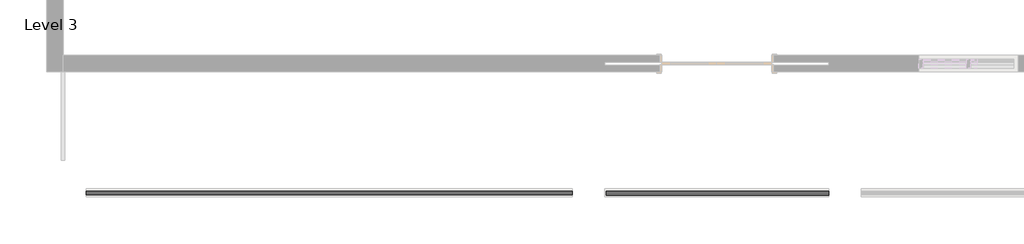
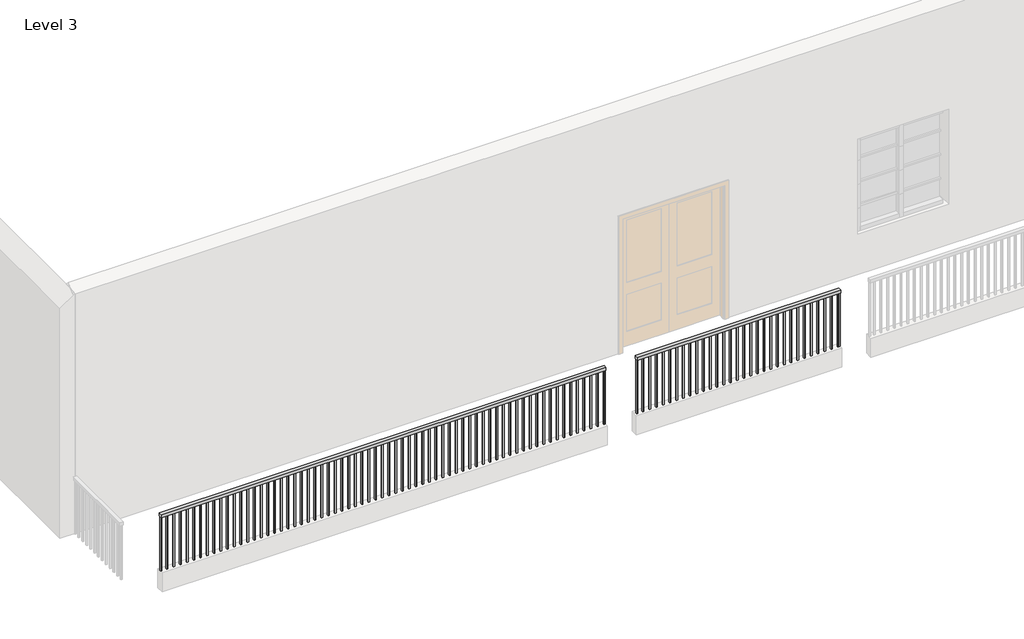
# One storey, part 2 of 3: 2 railings.
"""IFC4 building model written with IfcOpenShell, lengths in millimetres."""

from ifc_helpers import new_model, si_unit, frame, origin, place, context, project, spatial, polyline, outline, extrude, element, save

model = new_model("IFC4")

# Units and contexts
model_context = context("Model", 3, world=origin())
ifc_project = project(units=[si_unit("LENGTHUNIT", "METRE", prefix="MILLI")], contexts=[model_context])

# Site, building, storey
site = spatial("IfcSite", under=ifc_project)
building = spatial("IfcBuilding", under=site)
storey = spatial("IfcBuildingStorey", under=building, Name="Level 3", Elevation=3810.0)

# Railings
placement = place(None, origin())
element("IfcRailing", 1, ObjectType="Handrail - Rectangular", at=placement, inside=storey, context=model_context, shape_type="SweptSolid", body=[
    extrude(outline(polyline([(-9224.3420659, -8800.5902135), (-9224.3420659, -8749.7902135), (-2506.0420659, -8749.7902135), (-2506.0420659, -8800.5902135), (-9224.3420659, -8800.5902135)])), frame((0.0, 0.0, 4978.4), z_axis=(0.0, 0.0, 1.0), x_axis=(1.0, 0.0, 0.0)), (0.0, 0.0, 1.0), 50.8),
    extrude(outline(polyline([(-2528.2670659, -8784.7152135), (-2528.2670659, -8765.6652135), (-2509.2170659, -8765.6652135), (-2509.2170659, -8784.7152135), (-2528.2670659, -8784.7152135)])), frame((0.0, 0.0, 4114.8), z_axis=(0.0, 0.0, 1.0), x_axis=(1.0, 0.0, 0.0)), (0.0, 0.0, 1.0), 863.6),
    extrude(outline(polyline([(-2629.8670659, -8784.7152135), (-2629.8670659, -8765.6652135), (-2610.8170659, -8765.6652135), (-2610.8170659, -8784.7152135), (-2629.8670659, -8784.7152135)])), frame((0.0, 0.0, 4114.8), z_axis=(0.0, 0.0, 1.0), x_axis=(1.0, 0.0, 0.0)), (0.0, 0.0, 1.0), 863.6),
    extrude(outline(polyline([(-2731.4670659, -8784.7152135), (-2731.4670659, -8765.6652135), (-2712.4170659, -8765.6652135), (-2712.4170659, -8784.7152135), (-2731.4670659, -8784.7152135)])), frame((0.0, 0.0, 4114.8), z_axis=(0.0, 0.0, 1.0), x_axis=(1.0, 0.0, 0.0)), (0.0, 0.0, 1.0), 863.6),
    extrude(outline(polyline([(-2833.0670659, -8784.7152135), (-2833.0670659, -8765.6652135), (-2814.0170659, -8765.6652135), (-2814.0170659, -8784.7152135), (-2833.0670659, -8784.7152135)])), frame((0.0, 0.0, 4114.8), z_axis=(0.0, 0.0, 1.0), x_axis=(1.0, 0.0, 0.0)), (0.0, 0.0, 1.0), 863.6),
    extrude(outline(polyline([(-2934.6670659, -8784.7152135), (-2934.6670659, -8765.6652135), (-2915.6170659, -8765.6652135), (-2915.6170659, -8784.7152135), (-2934.6670659, -8784.7152135)])), frame((0.0, 0.0, 4114.8), z_axis=(0.0, 0.0, 1.0), x_axis=(1.0, 0.0, 0.0)), (0.0, 0.0, 1.0), 863.6),
    extrude(outline(polyline([(-3036.2670659, -8784.7152135), (-3036.2670659, -8765.6652135), (-3017.2170659, -8765.6652135), (-3017.2170659, -8784.7152135), (-3036.2670659, -8784.7152135)])), frame((0.0, 0.0, 4114.8), z_axis=(0.0, 0.0, 1.0), x_axis=(1.0, 0.0, 0.0)), (0.0, 0.0, 1.0), 863.6),
    extrude(outline(polyline([(-3137.8670659, -8784.7152135), (-3137.8670659, -8765.6652135), (-3118.8170659, -8765.6652135), (-3118.8170659, -8784.7152135), (-3137.8670659, -8784.7152135)])), frame((0.0, 0.0, 4114.8), z_axis=(0.0, 0.0, 1.0), x_axis=(1.0, 0.0, 0.0)), (0.0, 0.0, 1.0), 863.6),
    extrude(outline(polyline([(-3239.4670659, -8784.7152135), (-3239.4670659, -8765.6652135), (-3220.4170659, -8765.6652135), (-3220.4170659, -8784.7152135), (-3239.4670659, -8784.7152135)])), frame((0.0, 0.0, 4114.8), z_axis=(0.0, 0.0, 1.0), x_axis=(1.0, 0.0, 0.0)), (0.0, 0.0, 1.0), 863.6),
    extrude(outline(polyline([(-3341.0670659, -8784.7152135), (-3341.0670659, -8765.6652135), (-3322.0170659, -8765.6652135), (-3322.0170659, -8784.7152135), (-3341.0670659, -8784.7152135)])), frame((0.0, 0.0, 4114.8), z_axis=(0.0, 0.0, 1.0), x_axis=(1.0, 0.0, 0.0)), (0.0, 0.0, 1.0), 863.6),
    extrude(outline(polyline([(-3442.6670659, -8784.7152135), (-3442.6670659, -8765.6652135), (-3423.6170659, -8765.6652135), (-3423.6170659, -8784.7152135), (-3442.6670659, -8784.7152135)])), frame((0.0, 0.0, 4114.8), z_axis=(0.0, 0.0, 1.0), x_axis=(1.0, 0.0, 0.0)), (0.0, 0.0, 1.0), 863.6),
    extrude(outline(polyline([(-3544.2670659, -8784.7152135), (-3544.2670659, -8765.6652135), (-3525.2170659, -8765.6652135), (-3525.2170659, -8784.7152135), (-3544.2670659, -8784.7152135)])), frame((0.0, 0.0, 4114.8), z_axis=(0.0, 0.0, 1.0), x_axis=(1.0, 0.0, 0.0)), (0.0, 0.0, 1.0), 863.6),
    extrude(outline(polyline([(-3645.8670659, -8784.7152135), (-3645.8670659, -8765.6652135), (-3626.8170659, -8765.6652135), (-3626.8170659, -8784.7152135), (-3645.8670659, -8784.7152135)])), frame((0.0, 0.0, 4114.8), z_axis=(0.0, 0.0, 1.0), x_axis=(1.0, 0.0, 0.0)), (0.0, 0.0, 1.0), 863.6),
    extrude(outline(polyline([(-3747.4670659, -8784.7152135), (-3747.4670659, -8765.6652135), (-3728.4170659, -8765.6652135), (-3728.4170659, -8784.7152135), (-3747.4670659, -8784.7152135)])), frame((0.0, 0.0, 4114.8), z_axis=(0.0, 0.0, 1.0), x_axis=(1.0, 0.0, 0.0)), (0.0, 0.0, 1.0), 863.6),
    extrude(outline(polyline([(-3849.0670659, -8784.7152135), (-3849.0670659, -8765.6652135), (-3830.0170659, -8765.6652135), (-3830.0170659, -8784.7152135), (-3849.0670659, -8784.7152135)])), frame((0.0, 0.0, 4114.8), z_axis=(0.0, 0.0, 1.0), x_axis=(1.0, 0.0, 0.0)), (0.0, 0.0, 1.0), 863.6),
    extrude(outline(polyline([(-3950.6670659, -8784.7152135), (-3950.6670659, -8765.6652135), (-3931.6170659, -8765.6652135), (-3931.6170659, -8784.7152135), (-3950.6670659, -8784.7152135)])), frame((0.0, 0.0, 4114.8), z_axis=(0.0, 0.0, 1.0), x_axis=(1.0, 0.0, 0.0)), (0.0, 0.0, 1.0), 863.6),
    extrude(outline(polyline([(-4052.2670659, -8784.7152135), (-4052.2670659, -8765.6652135), (-4033.2170659, -8765.6652135), (-4033.2170659, -8784.7152135), (-4052.2670659, -8784.7152135)])), frame((0.0, 0.0, 4114.8), z_axis=(0.0, 0.0, 1.0), x_axis=(1.0, 0.0, 0.0)), (0.0, 0.0, 1.0), 863.6),
    extrude(outline(polyline([(-4153.8670659, -8784.7152135), (-4153.8670659, -8765.6652135), (-4134.8170659, -8765.6652135), (-4134.8170659, -8784.7152135), (-4153.8670659, -8784.7152135)])), frame((0.0, 0.0, 4114.8), z_axis=(0.0, 0.0, 1.0), x_axis=(1.0, 0.0, 0.0)), (0.0, 0.0, 1.0), 863.6),
    extrude(outline(polyline([(-4255.4670659, -8784.7152135), (-4255.4670659, -8765.6652135), (-4236.4170659, -8765.6652135), (-4236.4170659, -8784.7152135), (-4255.4670659, -8784.7152135)])), frame((0.0, 0.0, 4114.8), z_axis=(0.0, 0.0, 1.0), x_axis=(1.0, 0.0, 0.0)), (0.0, 0.0, 1.0), 863.6),
    extrude(outline(polyline([(-4357.0670659, -8784.7152135), (-4357.0670659, -8765.6652135), (-4338.0170659, -8765.6652135), (-4338.0170659, -8784.7152135), (-4357.0670659, -8784.7152135)])), frame((0.0, 0.0, 4114.8), z_axis=(0.0, 0.0, 1.0), x_axis=(1.0, 0.0, 0.0)), (0.0, 0.0, 1.0), 863.6),
    extrude(outline(polyline([(-4458.6670659, -8784.7152135), (-4458.6670659, -8765.6652135), (-4439.6170659, -8765.6652135), (-4439.6170659, -8784.7152135), (-4458.6670659, -8784.7152135)])), frame((0.0, 0.0, 4114.8), z_axis=(0.0, 0.0, 1.0), x_axis=(1.0, 0.0, 0.0)), (0.0, 0.0, 1.0), 863.6),
    extrude(outline(polyline([(-4560.2670659, -8784.7152135), (-4560.2670659, -8765.6652135), (-4541.2170659, -8765.6652135), (-4541.2170659, -8784.7152135), (-4560.2670659, -8784.7152135)])), frame((0.0, 0.0, 4114.8), z_axis=(0.0, 0.0, 1.0), x_axis=(1.0, 0.0, 0.0)), (0.0, 0.0, 1.0), 863.6),
    extrude(outline(polyline([(-4661.8670659, -8784.7152135), (-4661.8670659, -8765.6652135), (-4642.8170659, -8765.6652135), (-4642.8170659, -8784.7152135), (-4661.8670659, -8784.7152135)])), frame((0.0, 0.0, 4114.8), z_axis=(0.0, 0.0, 1.0), x_axis=(1.0, 0.0, 0.0)), (0.0, 0.0, 1.0), 863.6),
    extrude(outline(polyline([(-4763.4670659, -8784.7152135), (-4763.4670659, -8765.6652135), (-4744.4170659, -8765.6652135), (-4744.4170659, -8784.7152135), (-4763.4670659, -8784.7152135)])), frame((0.0, 0.0, 4114.8), z_axis=(0.0, 0.0, 1.0), x_axis=(1.0, 0.0, 0.0)), (0.0, 0.0, 1.0), 863.6),
    extrude(outline(polyline([(-4865.0670659, -8784.7152135), (-4865.0670659, -8765.6652135), (-4846.0170659, -8765.6652135), (-4846.0170659, -8784.7152135), (-4865.0670659, -8784.7152135)])), frame((0.0, 0.0, 4114.8), z_axis=(0.0, 0.0, 1.0), x_axis=(1.0, 0.0, 0.0)), (0.0, 0.0, 1.0), 863.6),
    extrude(outline(polyline([(-4966.6670659, -8784.7152135), (-4966.6670659, -8765.6652135), (-4947.6170659, -8765.6652135), (-4947.6170659, -8784.7152135), (-4966.6670659, -8784.7152135)])), frame((0.0, 0.0, 4114.8), z_axis=(0.0, 0.0, 1.0), x_axis=(1.0, 0.0, 0.0)), (0.0, 0.0, 1.0), 863.6),
    extrude(outline(polyline([(-5068.2670659, -8784.7152135), (-5068.2670659, -8765.6652135), (-5049.2170659, -8765.6652135), (-5049.2170659, -8784.7152135), (-5068.2670659, -8784.7152135)])), frame((0.0, 0.0, 4114.8), z_axis=(0.0, 0.0, 1.0), x_axis=(1.0, 0.0, 0.0)), (0.0, 0.0, 1.0), 863.6),
    extrude(outline(polyline([(-5169.8670659, -8784.7152135), (-5169.8670659, -8765.6652135), (-5150.8170659, -8765.6652135), (-5150.8170659, -8784.7152135), (-5169.8670659, -8784.7152135)])), frame((0.0, 0.0, 4114.8), z_axis=(0.0, 0.0, 1.0), x_axis=(1.0, 0.0, 0.0)), (0.0, 0.0, 1.0), 863.6),
    extrude(outline(polyline([(-5271.4670659, -8784.7152135), (-5271.4670659, -8765.6652135), (-5252.4170659, -8765.6652135), (-5252.4170659, -8784.7152135), (-5271.4670659, -8784.7152135)])), frame((0.0, 0.0, 4114.8), z_axis=(0.0, 0.0, 1.0), x_axis=(1.0, 0.0, 0.0)), (0.0, 0.0, 1.0), 863.6),
    extrude(outline(polyline([(-5373.0670659, -8784.7152135), (-5373.0670659, -8765.6652135), (-5354.0170659, -8765.6652135), (-5354.0170659, -8784.7152135), (-5373.0670659, -8784.7152135)])), frame((0.0, 0.0, 4114.8), z_axis=(0.0, 0.0, 1.0), x_axis=(1.0, 0.0, 0.0)), (0.0, 0.0, 1.0), 863.6),
    extrude(outline(polyline([(-5474.6670659, -8784.7152135), (-5474.6670659, -8765.6652135), (-5455.6170659, -8765.6652135), (-5455.6170659, -8784.7152135), (-5474.6670659, -8784.7152135)])), frame((0.0, 0.0, 4114.8), z_axis=(0.0, 0.0, 1.0), x_axis=(1.0, 0.0, 0.0)), (0.0, 0.0, 1.0), 863.6),
    extrude(outline(polyline([(-5576.2670659, -8784.7152135), (-5576.2670659, -8765.6652135), (-5557.2170659, -8765.6652135), (-5557.2170659, -8784.7152135), (-5576.2670659, -8784.7152135)])), frame((0.0, 0.0, 4114.8), z_axis=(0.0, 0.0, 1.0), x_axis=(1.0, 0.0, 0.0)), (0.0, 0.0, 1.0), 863.6),
    extrude(outline(polyline([(-5677.8670659, -8784.7152135), (-5677.8670659, -8765.6652135), (-5658.8170659, -8765.6652135), (-5658.8170659, -8784.7152135), (-5677.8670659, -8784.7152135)])), frame((0.0, 0.0, 4114.8), z_axis=(0.0, 0.0, 1.0), x_axis=(1.0, 0.0, 0.0)), (0.0, 0.0, 1.0), 863.6),
    extrude(outline(polyline([(-5779.4670659, -8784.7152135), (-5779.4670659, -8765.6652135), (-5760.4170659, -8765.6652135), (-5760.4170659, -8784.7152135), (-5779.4670659, -8784.7152135)])), frame((0.0, 0.0, 4114.8), z_axis=(0.0, 0.0, 1.0), x_axis=(1.0, 0.0, 0.0)), (0.0, 0.0, 1.0), 863.6),
    extrude(outline(polyline([(-5881.0670659, -8784.7152135), (-5881.0670659, -8765.6652135), (-5862.0170659, -8765.6652135), (-5862.0170659, -8784.7152135), (-5881.0670659, -8784.7152135)])), frame((0.0, 0.0, 4114.8), z_axis=(0.0, 0.0, 1.0), x_axis=(1.0, 0.0, 0.0)), (0.0, 0.0, 1.0), 863.6),
    extrude(outline(polyline([(-5982.6670659, -8784.7152135), (-5982.6670659, -8765.6652135), (-5963.6170659, -8765.6652135), (-5963.6170659, -8784.7152135), (-5982.6670659, -8784.7152135)])), frame((0.0, 0.0, 4114.8), z_axis=(0.0, 0.0, 1.0), x_axis=(1.0, 0.0, 0.0)), (0.0, 0.0, 1.0), 863.6),
    extrude(outline(polyline([(-6084.2670659, -8784.7152135), (-6084.2670659, -8765.6652135), (-6065.2170659, -8765.6652135), (-6065.2170659, -8784.7152135), (-6084.2670659, -8784.7152135)])), frame((0.0, 0.0, 4114.8), z_axis=(0.0, 0.0, 1.0), x_axis=(1.0, 0.0, 0.0)), (0.0, 0.0, 1.0), 863.6),
    extrude(outline(polyline([(-6185.8670659, -8784.7152135), (-6185.8670659, -8765.6652135), (-6166.8170659, -8765.6652135), (-6166.8170659, -8784.7152135), (-6185.8670659, -8784.7152135)])), frame((0.0, 0.0, 4114.8), z_axis=(0.0, 0.0, 1.0), x_axis=(1.0, 0.0, 0.0)), (0.0, 0.0, 1.0), 863.6),
    extrude(outline(polyline([(-6287.4670659, -8784.7152135), (-6287.4670659, -8765.6652135), (-6268.4170659, -8765.6652135), (-6268.4170659, -8784.7152135), (-6287.4670659, -8784.7152135)])), frame((0.0, 0.0, 4114.8), z_axis=(0.0, 0.0, 1.0), x_axis=(1.0, 0.0, 0.0)), (0.0, 0.0, 1.0), 863.6),
    extrude(outline(polyline([(-6389.0670659, -8784.7152135), (-6389.0670659, -8765.6652135), (-6370.0170659, -8765.6652135), (-6370.0170659, -8784.7152135), (-6389.0670659, -8784.7152135)])), frame((0.0, 0.0, 4114.8), z_axis=(0.0, 0.0, 1.0), x_axis=(1.0, 0.0, 0.0)), (0.0, 0.0, 1.0), 863.6),
    extrude(outline(polyline([(-6490.6670659, -8784.7152135), (-6490.6670659, -8765.6652135), (-6471.6170659, -8765.6652135), (-6471.6170659, -8784.7152135), (-6490.6670659, -8784.7152135)])), frame((0.0, 0.0, 4114.8), z_axis=(0.0, 0.0, 1.0), x_axis=(1.0, 0.0, 0.0)), (0.0, 0.0, 1.0), 863.6),
    extrude(outline(polyline([(-6592.2670659, -8784.7152135), (-6592.2670659, -8765.6652135), (-6573.2170659, -8765.6652135), (-6573.2170659, -8784.7152135), (-6592.2670659, -8784.7152135)])), frame((0.0, 0.0, 4114.8), z_axis=(0.0, 0.0, 1.0), x_axis=(1.0, 0.0, 0.0)), (0.0, 0.0, 1.0), 863.6),
    extrude(outline(polyline([(-6693.8670659, -8784.7152135), (-6693.8670659, -8765.6652135), (-6674.8170659, -8765.6652135), (-6674.8170659, -8784.7152135), (-6693.8670659, -8784.7152135)])), frame((0.0, 0.0, 4114.8), z_axis=(0.0, 0.0, 1.0), x_axis=(1.0, 0.0, 0.0)), (0.0, 0.0, 1.0), 863.6),
    extrude(outline(polyline([(-6795.4670659, -8784.7152135), (-6795.4670659, -8765.6652135), (-6776.4170659, -8765.6652135), (-6776.4170659, -8784.7152135), (-6795.4670659, -8784.7152135)])), frame((0.0, 0.0, 4114.8), z_axis=(0.0, 0.0, 1.0), x_axis=(1.0, 0.0, 0.0)), (0.0, 0.0, 1.0), 863.6),
    extrude(outline(polyline([(-6897.0670659, -8784.7152135), (-6897.0670659, -8765.6652135), (-6878.0170659, -8765.6652135), (-6878.0170659, -8784.7152135), (-6897.0670659, -8784.7152135)])), frame((0.0, 0.0, 4114.8), z_axis=(0.0, 0.0, 1.0), x_axis=(1.0, 0.0, 0.0)), (0.0, 0.0, 1.0), 863.6),
    extrude(outline(polyline([(-6998.6670659, -8784.7152135), (-6998.6670659, -8765.6652135), (-6979.6170659, -8765.6652135), (-6979.6170659, -8784.7152135), (-6998.6670659, -8784.7152135)])), frame((0.0, 0.0, 4114.8), z_axis=(0.0, 0.0, 1.0), x_axis=(1.0, 0.0, 0.0)), (0.0, 0.0, 1.0), 863.6),
    extrude(outline(polyline([(-7100.2670659, -8784.7152135), (-7100.2670659, -8765.6652135), (-7081.2170659, -8765.6652135), (-7081.2170659, -8784.7152135), (-7100.2670659, -8784.7152135)])), frame((0.0, 0.0, 4114.8), z_axis=(0.0, 0.0, 1.0), x_axis=(1.0, 0.0, 0.0)), (0.0, 0.0, 1.0), 863.6),
    extrude(outline(polyline([(-7201.8670659, -8784.7152135), (-7201.8670659, -8765.6652135), (-7182.8170659, -8765.6652135), (-7182.8170659, -8784.7152135), (-7201.8670659, -8784.7152135)])), frame((0.0, 0.0, 4114.8), z_axis=(0.0, 0.0, 1.0), x_axis=(1.0, 0.0, 0.0)), (0.0, 0.0, 1.0), 863.6),
    extrude(outline(polyline([(-7303.4670659, -8784.7152135), (-7303.4670659, -8765.6652135), (-7284.4170659, -8765.6652135), (-7284.4170659, -8784.7152135), (-7303.4670659, -8784.7152135)])), frame((0.0, 0.0, 4114.8), z_axis=(0.0, 0.0, 1.0), x_axis=(1.0, 0.0, 0.0)), (0.0, 0.0, 1.0), 863.6),
    extrude(outline(polyline([(-7405.0670659, -8784.7152135), (-7405.0670659, -8765.6652135), (-7386.0170659, -8765.6652135), (-7386.0170659, -8784.7152135), (-7405.0670659, -8784.7152135)])), frame((0.0, 0.0, 4114.8), z_axis=(0.0, 0.0, 1.0), x_axis=(1.0, 0.0, 0.0)), (0.0, 0.0, 1.0), 863.6),
    extrude(outline(polyline([(-7506.6670659, -8784.7152135), (-7506.6670659, -8765.6652135), (-7487.6170659, -8765.6652135), (-7487.6170659, -8784.7152135), (-7506.6670659, -8784.7152135)])), frame((0.0, 0.0, 4114.8), z_axis=(0.0, 0.0, 1.0), x_axis=(1.0, 0.0, 0.0)), (0.0, 0.0, 1.0), 863.6),
    extrude(outline(polyline([(-7608.2670659, -8784.7152135), (-7608.2670659, -8765.6652135), (-7589.2170659, -8765.6652135), (-7589.2170659, -8784.7152135), (-7608.2670659, -8784.7152135)])), frame((0.0, 0.0, 4114.8), z_axis=(0.0, 0.0, 1.0), x_axis=(1.0, 0.0, 0.0)), (0.0, 0.0, 1.0), 863.6),
    extrude(outline(polyline([(-7709.8670659, -8784.7152135), (-7709.8670659, -8765.6652135), (-7690.8170659, -8765.6652135), (-7690.8170659, -8784.7152135), (-7709.8670659, -8784.7152135)])), frame((0.0, 0.0, 4114.8), z_axis=(0.0, 0.0, 1.0), x_axis=(1.0, 0.0, 0.0)), (0.0, 0.0, 1.0), 863.6),
    extrude(outline(polyline([(-7811.4670659, -8784.7152135), (-7811.4670659, -8765.6652135), (-7792.4170659, -8765.6652135), (-7792.4170659, -8784.7152135), (-7811.4670659, -8784.7152135)])), frame((0.0, 0.0, 4114.8), z_axis=(0.0, 0.0, 1.0), x_axis=(1.0, 0.0, 0.0)), (0.0, 0.0, 1.0), 863.6),
    extrude(outline(polyline([(-7913.0670659, -8784.7152135), (-7913.0670659, -8765.6652135), (-7894.0170659, -8765.6652135), (-7894.0170659, -8784.7152135), (-7913.0670659, -8784.7152135)])), frame((0.0, 0.0, 4114.8), z_axis=(0.0, 0.0, 1.0), x_axis=(1.0, 0.0, 0.0)), (0.0, 0.0, 1.0), 863.6),
    extrude(outline(polyline([(-8014.6670659, -8784.7152135), (-8014.6670659, -8765.6652135), (-7995.6170659, -8765.6652135), (-7995.6170659, -8784.7152135), (-8014.6670659, -8784.7152135)])), frame((0.0, 0.0, 4114.8), z_axis=(0.0, 0.0, 1.0), x_axis=(1.0, 0.0, 0.0)), (0.0, 0.0, 1.0), 863.6),
    extrude(outline(polyline([(-8116.2670659, -8784.7152135), (-8116.2670659, -8765.6652135), (-8097.2170659, -8765.6652135), (-8097.2170659, -8784.7152135), (-8116.2670659, -8784.7152135)])), frame((0.0, 0.0, 4114.8), z_axis=(0.0, 0.0, 1.0), x_axis=(1.0, 0.0, 0.0)), (0.0, 0.0, 1.0), 863.6),
    extrude(outline(polyline([(-8217.8670659, -8784.7152135), (-8217.8670659, -8765.6652135), (-8198.8170659, -8765.6652135), (-8198.8170659, -8784.7152135), (-8217.8670659, -8784.7152135)])), frame((0.0, 0.0, 4114.8), z_axis=(0.0, 0.0, 1.0), x_axis=(1.0, 0.0, 0.0)), (0.0, 0.0, 1.0), 863.6),
    extrude(outline(polyline([(-8319.4670659, -8784.7152135), (-8319.4670659, -8765.6652135), (-8300.4170659, -8765.6652135), (-8300.4170659, -8784.7152135), (-8319.4670659, -8784.7152135)])), frame((0.0, 0.0, 4114.8), z_axis=(0.0, 0.0, 1.0), x_axis=(1.0, 0.0, 0.0)), (0.0, 0.0, 1.0), 863.6),
    extrude(outline(polyline([(-8421.0670659, -8784.7152135), (-8421.0670659, -8765.6652135), (-8402.0170659, -8765.6652135), (-8402.0170659, -8784.7152135), (-8421.0670659, -8784.7152135)])), frame((0.0, 0.0, 4114.8), z_axis=(0.0, 0.0, 1.0), x_axis=(1.0, 0.0, 0.0)), (0.0, 0.0, 1.0), 863.6),
    extrude(outline(polyline([(-8522.6670659, -8784.7152135), (-8522.6670659, -8765.6652135), (-8503.6170659, -8765.6652135), (-8503.6170659, -8784.7152135), (-8522.6670659, -8784.7152135)])), frame((0.0, 0.0, 4114.8), z_axis=(0.0, 0.0, 1.0), x_axis=(1.0, 0.0, 0.0)), (0.0, 0.0, 1.0), 863.6),
    extrude(outline(polyline([(-8624.2670659, -8784.7152135), (-8624.2670659, -8765.6652135), (-8605.2170659, -8765.6652135), (-8605.2170659, -8784.7152135), (-8624.2670659, -8784.7152135)])), frame((0.0, 0.0, 4114.8), z_axis=(0.0, 0.0, 1.0), x_axis=(1.0, 0.0, 0.0)), (0.0, 0.0, 1.0), 863.6),
    extrude(outline(polyline([(-8725.8670659, -8784.7152135), (-8725.8670659, -8765.6652135), (-8706.8170659, -8765.6652135), (-8706.8170659, -8784.7152135), (-8725.8670659, -8784.7152135)])), frame((0.0, 0.0, 4114.8), z_axis=(0.0, 0.0, 1.0), x_axis=(1.0, 0.0, 0.0)), (0.0, 0.0, 1.0), 863.6),
    extrude(outline(polyline([(-8827.4670659, -8784.7152135), (-8827.4670659, -8765.6652135), (-8808.4170659, -8765.6652135), (-8808.4170659, -8784.7152135), (-8827.4670659, -8784.7152135)])), frame((0.0, 0.0, 4114.8), z_axis=(0.0, 0.0, 1.0), x_axis=(1.0, 0.0, 0.0)), (0.0, 0.0, 1.0), 863.6),
    extrude(outline(polyline([(-8929.0670659, -8784.7152135), (-8929.0670659, -8765.6652135), (-8910.0170659, -8765.6652135), (-8910.0170659, -8784.7152135), (-8929.0670659, -8784.7152135)])), frame((0.0, 0.0, 4114.8), z_axis=(0.0, 0.0, 1.0), x_axis=(1.0, 0.0, 0.0)), (0.0, 0.0, 1.0), 863.6),
    extrude(outline(polyline([(-9030.6670659, -8784.7152135), (-9030.6670659, -8765.6652135), (-9011.6170659, -8765.6652135), (-9011.6170659, -8784.7152135), (-9030.6670659, -8784.7152135)])), frame((0.0, 0.0, 4114.8), z_axis=(0.0, 0.0, 1.0), x_axis=(1.0, 0.0, 0.0)), (0.0, 0.0, 1.0), 863.6),
    extrude(outline(polyline([(-9132.2670659, -8784.7152135), (-9132.2670659, -8765.6652135), (-9113.2170659, -8765.6652135), (-9113.2170659, -8784.7152135), (-9132.2670659, -8784.7152135)])), frame((0.0, 0.0, 4114.8), z_axis=(0.0, 0.0, 1.0), x_axis=(1.0, 0.0, 0.0)), (0.0, 0.0, 1.0), 863.6),
    extrude(outline(polyline([(-2525.0920659, -8784.7152135), (-2525.0920659, -8765.6652135), (-2506.0420659, -8765.6652135), (-2506.0420659, -8784.7152135), (-2525.0920659, -8784.7152135)])), frame((0.0, 0.0, 4114.8), z_axis=(0.0, 0.0, 1.0), x_axis=(1.0, 0.0, 0.0)), (0.0, 0.0, 1.0), 863.6),
    extrude(outline(polyline([(-9224.3420659, -8784.7152135), (-9224.3420659, -8765.6652135), (-9205.2920659, -8765.6652135), (-9205.2920659, -8784.7152135), (-9224.3420659, -8784.7152135)])), frame((0.0, 0.0, 4114.8), z_axis=(0.0, 0.0, 1.0), x_axis=(1.0, 0.0, 0.0)), (0.0, 0.0, 1.0), 863.6),
])
element("IfcRailing", 2, ObjectType="Handrail - Rectangular", at=placement, inside=storey, context=model_context, shape_type="SweptSolid", body=[
    extrude(outline(polyline([(-2036.1420659, -8802.2878342), (-2036.1420659, -8751.4878342), (1037.2579341, -8751.4878342), (1037.2579341, -8802.2878342), (-2036.1420659, -8802.2878342)])), frame((0.0, 0.0, 4978.4), z_axis=(0.0, 0.0, 1.0), x_axis=(1.0, 0.0, 0.0)), (0.0, 0.0, 1.0), 50.8),
    extrude(outline(polyline([(1002.3329341, -8786.4128342), (1002.3329341, -8767.3628342), (1021.3829341, -8767.3628342), (1021.3829341, -8786.4128342), (1002.3329341, -8786.4128342)])), frame((0.0, 0.0, 4114.8), z_axis=(0.0, 0.0, 1.0), x_axis=(1.0, 0.0, 0.0)), (0.0, 0.0, 1.0), 863.6),
    extrude(outline(polyline([(900.7329341, -8786.4128342), (900.7329341, -8767.3628342), (919.7829341, -8767.3628342), (919.7829341, -8786.4128342), (900.7329341, -8786.4128342)])), frame((0.0, 0.0, 4114.8), z_axis=(0.0, 0.0, 1.0), x_axis=(1.0, 0.0, 0.0)), (0.0, 0.0, 1.0), 863.6),
    extrude(outline(polyline([(799.1329341, -8786.4128342), (799.1329341, -8767.3628342), (818.1829341, -8767.3628342), (818.1829341, -8786.4128342), (799.1329341, -8786.4128342)])), frame((0.0, 0.0, 4114.8), z_axis=(0.0, 0.0, 1.0), x_axis=(1.0, 0.0, 0.0)), (0.0, 0.0, 1.0), 863.6),
    extrude(outline(polyline([(697.5329341, -8786.4128342), (697.5329341, -8767.3628342), (716.5829341, -8767.3628342), (716.5829341, -8786.4128342), (697.5329341, -8786.4128342)])), frame((0.0, 0.0, 4114.8), z_axis=(0.0, 0.0, 1.0), x_axis=(1.0, 0.0, 0.0)), (0.0, 0.0, 1.0), 863.6),
    extrude(outline(polyline([(595.9329341, -8786.4128342), (595.9329341, -8767.3628342), (614.9829341, -8767.3628342), (614.9829341, -8786.4128342), (595.9329341, -8786.4128342)])), frame((0.0, 0.0, 4114.8), z_axis=(0.0, 0.0, 1.0), x_axis=(1.0, 0.0, 0.0)), (0.0, 0.0, 1.0), 863.6),
    extrude(outline(polyline([(494.3329341, -8786.4128342), (494.3329341, -8767.3628342), (513.3829341, -8767.3628342), (513.3829341, -8786.4128342), (494.3329341, -8786.4128342)])), frame((0.0, 0.0, 4114.8), z_axis=(0.0, 0.0, 1.0), x_axis=(1.0, 0.0, 0.0)), (0.0, 0.0, 1.0), 863.6),
    extrude(outline(polyline([(392.7329341, -8786.4128342), (392.7329341, -8767.3628342), (411.7829341, -8767.3628342), (411.7829341, -8786.4128342), (392.7329341, -8786.4128342)])), frame((0.0, 0.0, 4114.8), z_axis=(0.0, 0.0, 1.0), x_axis=(1.0, 0.0, 0.0)), (0.0, 0.0, 1.0), 863.6),
    extrude(outline(polyline([(291.1329341, -8786.4128342), (291.1329341, -8767.3628342), (310.1829341, -8767.3628342), (310.1829341, -8786.4128342), (291.1329341, -8786.4128342)])), frame((0.0, 0.0, 4114.8), z_axis=(0.0, 0.0, 1.0), x_axis=(1.0, 0.0, 0.0)), (0.0, 0.0, 1.0), 863.6),
    extrude(outline(polyline([(189.5329341, -8786.4128342), (189.5329341, -8767.3628342), (208.5829341, -8767.3628342), (208.5829341, -8786.4128342), (189.5329341, -8786.4128342)])), frame((0.0, 0.0, 4114.8), z_axis=(0.0, 0.0, 1.0), x_axis=(1.0, 0.0, 0.0)), (0.0, 0.0, 1.0), 863.6),
    extrude(outline(polyline([(87.9329341, -8786.4128342), (87.9329341, -8767.3628342), (106.9829341, -8767.3628342), (106.9829341, -8786.4128342), (87.9329341, -8786.4128342)])), frame((0.0, 0.0, 4114.8), z_axis=(0.0, 0.0, 1.0), x_axis=(1.0, 0.0, 0.0)), (0.0, 0.0, 1.0), 863.6),
    extrude(outline(polyline([(-13.6670659, -8786.4128342), (-13.6670659, -8767.3628342), (5.3829341, -8767.3628342), (5.3829341, -8786.4128342), (-13.6670659, -8786.4128342)])), frame((0.0, 0.0, 4114.8), z_axis=(0.0, 0.0, 1.0), x_axis=(1.0, 0.0, 0.0)), (0.0, 0.0, 1.0), 863.6),
    extrude(outline(polyline([(-115.2670659, -8786.4128342), (-115.2670659, -8767.3628342), (-96.2170659, -8767.3628342), (-96.2170659, -8786.4128342), (-115.2670659, -8786.4128342)])), frame((0.0, 0.0, 4114.8), z_axis=(0.0, 0.0, 1.0), x_axis=(1.0, 0.0, 0.0)), (0.0, 0.0, 1.0), 863.6),
    extrude(outline(polyline([(-216.8670659, -8786.4128342), (-216.8670659, -8767.3628342), (-197.8170659, -8767.3628342), (-197.8170659, -8786.4128342), (-216.8670659, -8786.4128342)])), frame((0.0, 0.0, 4114.8), z_axis=(0.0, 0.0, 1.0), x_axis=(1.0, 0.0, 0.0)), (0.0, 0.0, 1.0), 863.6),
    extrude(outline(polyline([(-318.4670659, -8786.4128342), (-318.4670659, -8767.3628342), (-299.4170659, -8767.3628342), (-299.4170659, -8786.4128342), (-318.4670659, -8786.4128342)])), frame((0.0, 0.0, 4114.8), z_axis=(0.0, 0.0, 1.0), x_axis=(1.0, 0.0, 0.0)), (0.0, 0.0, 1.0), 863.6),
    extrude(outline(polyline([(-420.0670659, -8786.4128342), (-420.0670659, -8767.3628342), (-401.0170659, -8767.3628342), (-401.0170659, -8786.4128342), (-420.0670659, -8786.4128342)])), frame((0.0, 0.0, 4114.8), z_axis=(0.0, 0.0, 1.0), x_axis=(1.0, 0.0, 0.0)), (0.0, 0.0, 1.0), 863.6),
    extrude(outline(polyline([(-521.6670659, -8786.4128342), (-521.6670659, -8767.3628342), (-502.6170659, -8767.3628342), (-502.6170659, -8786.4128342), (-521.6670659, -8786.4128342)])), frame((0.0, 0.0, 4114.8), z_axis=(0.0, 0.0, 1.0), x_axis=(1.0, 0.0, 0.0)), (0.0, 0.0, 1.0), 863.6),
    extrude(outline(polyline([(-623.2670659, -8786.4128342), (-623.2670659, -8767.3628342), (-604.2170659, -8767.3628342), (-604.2170659, -8786.4128342), (-623.2670659, -8786.4128342)])), frame((0.0, 0.0, 4114.8), z_axis=(0.0, 0.0, 1.0), x_axis=(1.0, 0.0, 0.0)), (0.0, 0.0, 1.0), 863.6),
    extrude(outline(polyline([(-724.8670659, -8786.4128342), (-724.8670659, -8767.3628342), (-705.8170659, -8767.3628342), (-705.8170659, -8786.4128342), (-724.8670659, -8786.4128342)])), frame((0.0, 0.0, 4114.8), z_axis=(0.0, 0.0, 1.0), x_axis=(1.0, 0.0, 0.0)), (0.0, 0.0, 1.0), 863.6),
    extrude(outline(polyline([(-826.4670659, -8786.4128342), (-826.4670659, -8767.3628342), (-807.4170659, -8767.3628342), (-807.4170659, -8786.4128342), (-826.4670659, -8786.4128342)])), frame((0.0, 0.0, 4114.8), z_axis=(0.0, 0.0, 1.0), x_axis=(1.0, 0.0, 0.0)), (0.0, 0.0, 1.0), 863.6),
    extrude(outline(polyline([(-928.0670659, -8786.4128342), (-928.0670659, -8767.3628342), (-909.0170659, -8767.3628342), (-909.0170659, -8786.4128342), (-928.0670659, -8786.4128342)])), frame((0.0, 0.0, 4114.8), z_axis=(0.0, 0.0, 1.0), x_axis=(1.0, 0.0, 0.0)), (0.0, 0.0, 1.0), 863.6),
    extrude(outline(polyline([(-1029.6670659, -8786.4128342), (-1029.6670659, -8767.3628342), (-1010.6170659, -8767.3628342), (-1010.6170659, -8786.4128342), (-1029.6670659, -8786.4128342)])), frame((0.0, 0.0, 4114.8), z_axis=(0.0, 0.0, 1.0), x_axis=(1.0, 0.0, 0.0)), (0.0, 0.0, 1.0), 863.6),
    extrude(outline(polyline([(-1131.2670659, -8786.4128342), (-1131.2670659, -8767.3628342), (-1112.2170659, -8767.3628342), (-1112.2170659, -8786.4128342), (-1131.2670659, -8786.4128342)])), frame((0.0, 0.0, 4114.8), z_axis=(0.0, 0.0, 1.0), x_axis=(1.0, 0.0, 0.0)), (0.0, 0.0, 1.0), 863.6),
    extrude(outline(polyline([(-1232.8670659, -8786.4128342), (-1232.8670659, -8767.3628342), (-1213.8170659, -8767.3628342), (-1213.8170659, -8786.4128342), (-1232.8670659, -8786.4128342)])), frame((0.0, 0.0, 4114.8), z_axis=(0.0, 0.0, 1.0), x_axis=(1.0, 0.0, 0.0)), (0.0, 0.0, 1.0), 863.6),
    extrude(outline(polyline([(-1334.4670659, -8786.4128342), (-1334.4670659, -8767.3628342), (-1315.4170659, -8767.3628342), (-1315.4170659, -8786.4128342), (-1334.4670659, -8786.4128342)])), frame((0.0, 0.0, 4114.8), z_axis=(0.0, 0.0, 1.0), x_axis=(1.0, 0.0, 0.0)), (0.0, 0.0, 1.0), 863.6),
    extrude(outline(polyline([(-1436.0670659, -8786.4128342), (-1436.0670659, -8767.3628342), (-1417.0170659, -8767.3628342), (-1417.0170659, -8786.4128342), (-1436.0670659, -8786.4128342)])), frame((0.0, 0.0, 4114.8), z_axis=(0.0, 0.0, 1.0), x_axis=(1.0, 0.0, 0.0)), (0.0, 0.0, 1.0), 863.6),
    extrude(outline(polyline([(-1537.6670659, -8786.4128342), (-1537.6670659, -8767.3628342), (-1518.6170659, -8767.3628342), (-1518.6170659, -8786.4128342), (-1537.6670659, -8786.4128342)])), frame((0.0, 0.0, 4114.8), z_axis=(0.0, 0.0, 1.0), x_axis=(1.0, 0.0, 0.0)), (0.0, 0.0, 1.0), 863.6),
    extrude(outline(polyline([(-1639.2670659, -8786.4128342), (-1639.2670659, -8767.3628342), (-1620.2170659, -8767.3628342), (-1620.2170659, -8786.4128342), (-1639.2670659, -8786.4128342)])), frame((0.0, 0.0, 4114.8), z_axis=(0.0, 0.0, 1.0), x_axis=(1.0, 0.0, 0.0)), (0.0, 0.0, 1.0), 863.6),
    extrude(outline(polyline([(-1740.8670659, -8786.4128342), (-1740.8670659, -8767.3628342), (-1721.8170659, -8767.3628342), (-1721.8170659, -8786.4128342), (-1740.8670659, -8786.4128342)])), frame((0.0, 0.0, 4114.8), z_axis=(0.0, 0.0, 1.0), x_axis=(1.0, 0.0, 0.0)), (0.0, 0.0, 1.0), 863.6),
    extrude(outline(polyline([(-1842.4670659, -8786.4128342), (-1842.4670659, -8767.3628342), (-1823.4170659, -8767.3628342), (-1823.4170659, -8786.4128342), (-1842.4670659, -8786.4128342)])), frame((0.0, 0.0, 4114.8), z_axis=(0.0, 0.0, 1.0), x_axis=(1.0, 0.0, 0.0)), (0.0, 0.0, 1.0), 863.6),
    extrude(outline(polyline([(-1944.0670659, -8786.4128342), (-1944.0670659, -8767.3628342), (-1925.0170659, -8767.3628342), (-1925.0170659, -8786.4128342), (-1944.0670659, -8786.4128342)])), frame((0.0, 0.0, 4114.8), z_axis=(0.0, 0.0, 1.0), x_axis=(1.0, 0.0, 0.0)), (0.0, 0.0, 1.0), 863.6),
    extrude(outline(polyline([(1018.2079341, -8786.4128342), (1018.2079341, -8767.3628342), (1037.2579341, -8767.3628342), (1037.2579341, -8786.4128342), (1018.2079341, -8786.4128342)])), frame((0.0, 0.0, 4114.8), z_axis=(0.0, 0.0, 1.0), x_axis=(1.0, 0.0, 0.0)), (0.0, 0.0, 1.0), 863.6),
    extrude(outline(polyline([(-2036.1420659, -8786.4128342), (-2036.1420659, -8767.3628342), (-2017.0920659, -8767.3628342), (-2017.0920659, -8786.4128342), (-2036.1420659, -8786.4128342)])), frame((0.0, 0.0, 4114.8), z_axis=(0.0, 0.0, 1.0), x_axis=(1.0, 0.0, 0.0)), (0.0, 0.0, 1.0), 863.6),
])

save(model, "model.ifc")

# Revit data of these elements
# Type "Handrail - Rectangular"
#   Assembly Code = "C2010400"
#   built-in parameter 1008612 = 0.0416667 (stored number, unit not read)
#   built-in parameter 1008611 = 0.0416667 (stored number, unit not read)
#   built-in parameter 1008609 = 0.333333 (stored number, unit not read)
#   built-in parameter 1008604 = 0.166667 (stored number, unit not read)
#   built-in parameter 1008603 = 0.166667 (stored number, unit not read)
#   Railing Height = 3' - 0"
#   built-in parameter 1008630 = 2
#   built-in parameter 1008610 = 2
#   built-in parameter 1008618 = Baluster - Square : 3/4"
# Elements 1, 2 (IfcRailing, "Handrail - Rectangular")
#   built-in parameter 1008621 = 1 (stored number, unit not read)
#   Phase Created = New Construction
